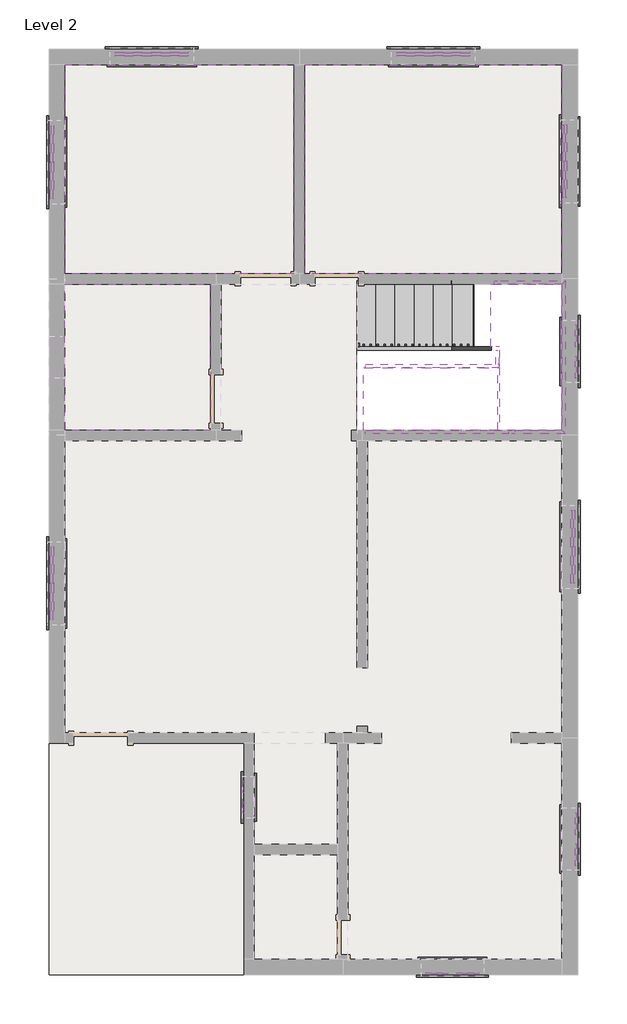
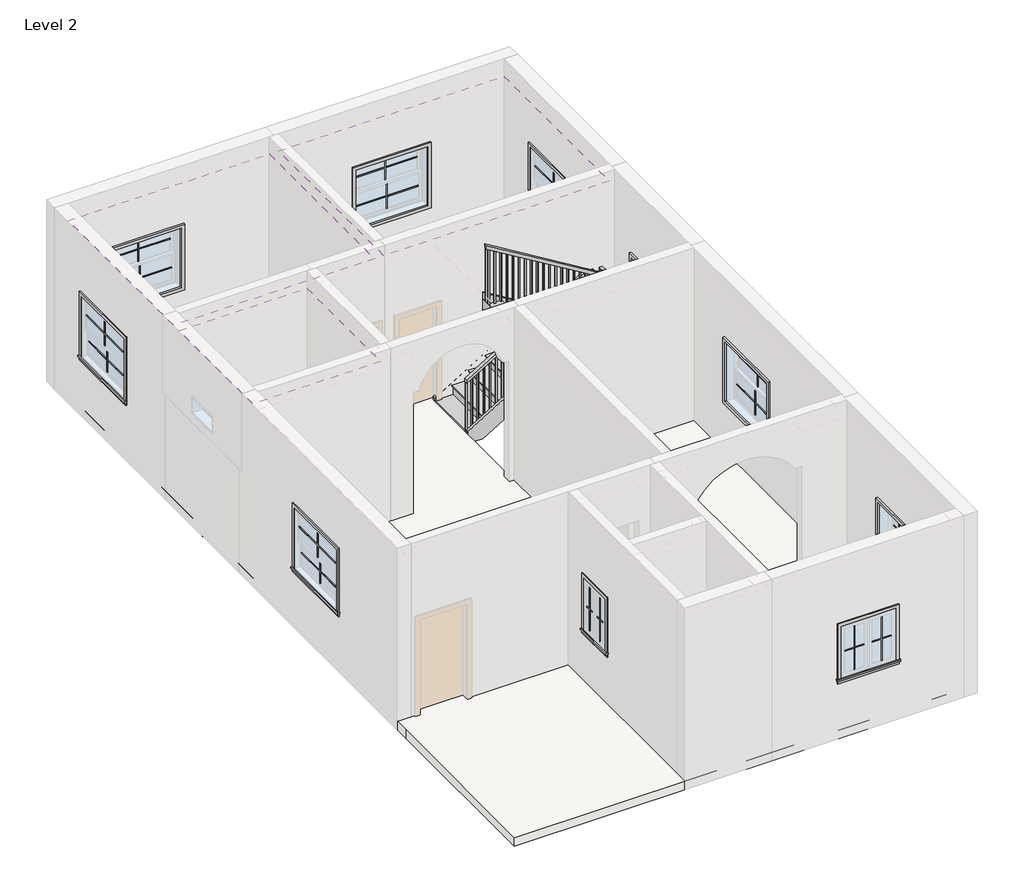
# One storey, part 2 of 2: 40 proxies, 8 members, 3 coverings, 2 slabs, 2 stair flights, 1 railing.
"""IFC4 building model written with IfcOpenShell, lengths in millimetres."""

from ifc_helpers import new_model, si_unit, frame, origin, place, context, project, spatial, polyline, outline, extrude, faceted_brep, transform, mapped, element, save
from components import muntin_pattern_2x2_muntin_pattern_2x2_8b3f23e7, muntin_pattern_2x2_muntin_pattern_2x2_5e52a1c6, muntin_pattern_2x2_muntin_pattern_2x2_d1c6e638, muntin_pattern_2x2_muntin_pattern_2x2_37b95fb2, muntin_pattern_2x2_muntin_pattern_2x2_53152e2c, muntin_pattern_2x2_muntin_pattern_2x2_e8f3e573, trim_window_exterior_flat_with_sill_f44f30ad, trim_window_exterior_flat_with_sill_e2e7eb1d, trim_window_exterior_flat_with_sill_84e24481, trim_window_exterior_flat_with_sill_a665a915, trim_window_interior_flat_picture_frame_1dce1945, trim_window_interior_flat_picture_frame_a40cb921, trim_window_interior_flat_picture_frame_28d4e5dc, trim_window_interior_flat_picture_frame_d485c387, non_monolithic_landing_52da1c58, stair_flight_171342da, stair_flight_f02a3465

model = new_model("IFC4")

# Units and contexts
model_context = context("Model", 3, world=origin())
ifc_project = project(units=[si_unit("LENGTHUNIT", "METRE", prefix="MILLI")], contexts=[model_context])

# Site, building, storey
site = spatial("IfcSite", under=ifc_project)
building = spatial("IfcBuilding", under=site)
storey = spatial("IfcBuildingStorey", under=building, Name="Level 2", Elevation=3200.4)

# Proxies
placement = place(None, origin())
muntin_pattern_2x2_muntin_pattern_2x2_shape = muntin_pattern_2x2_muntin_pattern_2x2_8b3f23e7(model_context)
element("IfcBuildingElementProxy", 1, Name="Muntin Pattern_2x2 : Muntin Pattern_2x2", ObjectType="Muntin Pattern_2x2 : Muntin Pattern_2x2", at=placement, inside=storey, context=model_context, shape_type="MappedRepresentation", body=[
    mapped(muntin_pattern_2x2_muntin_pattern_2x2_shape, transform((-5865.439062, 5032.1857363, 4975.225), x_axis=(0.0, 1.0, 0.0), y_axis=(-1.0, 0.0, 0.0), z_axis=(0.0, 0.0, 1.0))),
])
element("IfcBuildingElementProxy", 2, Name="Muntin Pattern_2x2 : Muntin Pattern_2x2", ObjectType="Muntin Pattern_2x2 : Muntin Pattern_2x2", at=placement, inside=storey, context=model_context, shape_type="MappedRepresentation", body=[
    mapped(muntin_pattern_2x2_muntin_pattern_2x2_shape, transform((-5820.989062, 5032.1857363, 4495.8), x_axis=(0.0, 1.0, 0.0), y_axis=(-1.0, 0.0, 0.0), z_axis=(0.0, 0.0, 1.0))),
])
element("IfcBuildingElementProxy", 3, Name="Muntin Pattern_2x2 : Muntin Pattern_2x2", ObjectType="Muntin Pattern_2x2 : Muntin Pattern_2x2", at=placement, inside=storey, context=model_context, shape_type="MappedRepresentation", body=[
    mapped(muntin_pattern_2x2_muntin_pattern_2x2_shape, transform((1786.310938, -581.2142637, 4975.225), x_axis=(0.0, -1.0, 0.0), y_axis=(1.0, 0.0, 0.0), z_axis=(0.0, 0.0, 1.0))),
])
element("IfcBuildingElementProxy", 4, Name="Muntin Pattern_2x2 : Muntin Pattern_2x2", ObjectType="Muntin Pattern_2x2 : Muntin Pattern_2x2", at=placement, inside=storey, context=model_context, shape_type="MappedRepresentation", body=[
    mapped(muntin_pattern_2x2_muntin_pattern_2x2_shape, transform((1741.860938, -581.2142637, 4495.8), x_axis=(0.0, -1.0, 0.0), y_axis=(1.0, 0.0, 0.0), z_axis=(0.0, 0.0, 1.0))),
])
element("IfcBuildingElementProxy", 5, Name="Muntin Pattern_2x2 : Muntin Pattern_2x2", ObjectType="Muntin Pattern_2x2 : Muntin Pattern_2x2", at=placement, inside=storey, context=model_context, shape_type="MappedRepresentation", body=[
    mapped(muntin_pattern_2x2_muntin_pattern_2x2_shape, transform((-5865.439062, -1114.6142637, 4975.225), x_axis=(0.0, 1.0, 0.0), y_axis=(-1.0, 0.0, 0.0), z_axis=(0.0, 0.0, 1.0))),
])
element("IfcBuildingElementProxy", 6, Name="Muntin Pattern_2x2 : Muntin Pattern_2x2", ObjectType="Muntin Pattern_2x2 : Muntin Pattern_2x2", at=placement, inside=storey, context=model_context, shape_type="MappedRepresentation", body=[
    mapped(muntin_pattern_2x2_muntin_pattern_2x2_shape, transform((-5820.989062, -1114.6142637, 4495.8), x_axis=(0.0, 1.0, 0.0), y_axis=(-1.0, 0.0, 0.0), z_axis=(0.0, 0.0, 1.0))),
])
muntin_pattern_2x2_muntin_pattern_2x2_2_shape = muntin_pattern_2x2_muntin_pattern_2x2_5e52a1c6(model_context)
element("IfcBuildingElementProxy", 7, Name="Muntin Pattern_2x2 : Muntin Pattern_2x2", ObjectType="Muntin Pattern_2x2 : Muntin Pattern_2x2", at=placement, inside=storey, context=model_context, shape_type="MappedRepresentation", body=[
    mapped(muntin_pattern_2x2_muntin_pattern_2x2_2_shape, transform((-4401.764062, 6648.2607363, 4975.225), x_axis=(-1.0, 0.0, 0.0), y_axis=(0.0, -1.0, 0.0), z_axis=(0.0, 0.0, 1.0))),
])
element("IfcBuildingElementProxy", 8, Name="Muntin Pattern_2x2 : Muntin Pattern_2x2", ObjectType="Muntin Pattern_2x2 : Muntin Pattern_2x2", at=placement, inside=storey, context=model_context, shape_type="MappedRepresentation", body=[
    mapped(muntin_pattern_2x2_muntin_pattern_2x2_2_shape, transform((-4401.764062, 6603.8107363, 4495.8), x_axis=(-1.0, 0.0, 0.0), y_axis=(0.0, -1.0, 0.0), z_axis=(0.0, 0.0, 1.0))),
])
element("IfcBuildingElementProxy", 9, Name="Muntin Pattern_2x2 : Muntin Pattern_2x2", ObjectType="Muntin Pattern_2x2 : Muntin Pattern_2x2", at=placement, inside=storey, context=model_context, shape_type="MappedRepresentation", body=[
    mapped(muntin_pattern_2x2_muntin_pattern_2x2_2_shape, transform((-286.964062, 6648.2607363, 4975.225), x_axis=(-1.0, 0.0, 0.0), y_axis=(0.0, -1.0, 0.0), z_axis=(0.0, 0.0, 1.0))),
])
element("IfcBuildingElementProxy", 10, Name="Muntin Pattern_2x2 : Muntin Pattern_2x2", ObjectType="Muntin Pattern_2x2 : Muntin Pattern_2x2", at=placement, inside=storey, context=model_context, shape_type="MappedRepresentation", body=[
    mapped(muntin_pattern_2x2_muntin_pattern_2x2_2_shape, transform((-286.964062, 6603.8107363, 4495.8), x_axis=(-1.0, 0.0, 0.0), y_axis=(0.0, -1.0, 0.0), z_axis=(0.0, 0.0, 1.0))),
])
element("IfcBuildingElementProxy", 11, Name="Muntin Pattern_2x2 : Muntin Pattern_2x2", ObjectType="Muntin Pattern_2x2 : Muntin Pattern_2x2", at=placement, inside=storey, context=model_context, shape_type="MappedRepresentation", body=[
    mapped(muntin_pattern_2x2_muntin_pattern_2x2_2_shape, transform((1627.560938, 5044.8857363, 4975.225), x_axis=(0.0, -1.0, 0.0), y_axis=(1.0, 0.0, 0.0), z_axis=(0.0, 0.0, 1.0))),
])
element("IfcBuildingElementProxy", 12, Name="Muntin Pattern_2x2 : Muntin Pattern_2x2", ObjectType="Muntin Pattern_2x2 : Muntin Pattern_2x2", at=placement, inside=storey, context=model_context, shape_type="MappedRepresentation", body=[
    mapped(muntin_pattern_2x2_muntin_pattern_2x2_2_shape, transform((1672.010938, 5044.8857363, 4495.8), x_axis=(0.0, -1.0, 0.0), y_axis=(1.0, 0.0, 0.0), z_axis=(0.0, 0.0, 1.0))),
])
muntin_pattern_2x2_muntin_pattern_2x2_3_shape = muntin_pattern_2x2_muntin_pattern_2x2_d1c6e638(model_context)
element("IfcBuildingElementProxy", 13, Name="Muntin Pattern_2x2 : Muntin Pattern_2x2", ObjectType="Muntin Pattern_2x2 : Muntin Pattern_2x2", at=placement, inside=storey, context=model_context, shape_type="MappedRepresentation", body=[
    mapped(muntin_pattern_2x2_muntin_pattern_2x2_3_shape, transform((1811.710938, -4621.4017637, 4489.45), x_axis=(0.0, -1.0, 0.0), y_axis=(1.0, 0.0, 0.0), z_axis=(0.0, 0.0, 1.0))),
])
element("IfcBuildingElementProxy", 14, Name="Muntin Pattern_2x2 : Muntin Pattern_2x2", ObjectType="Muntin Pattern_2x2 : Muntin Pattern_2x2", at=placement, inside=storey, context=model_context, shape_type="MappedRepresentation", body=[
    mapped(muntin_pattern_2x2_muntin_pattern_2x2_3_shape, transform((219.448438, -6820.0892637, 4489.45), x_axis=(-1.0, 0.0, 0.0), y_axis=(0.0, -1.0, 0.0), z_axis=(0.0, 0.0, 1.0))),
])
element("IfcBuildingElementProxy", 15, Name="Muntin Pattern_2x2 : Muntin Pattern_2x2", ObjectType="Muntin Pattern_2x2 : Muntin Pattern_2x2", at=placement, inside=storey, context=model_context, shape_type="MappedRepresentation", body=[
    mapped(muntin_pattern_2x2_muntin_pattern_2x2_3_shape, transform((1811.710938, 2496.9482363, 4489.45), x_axis=(0.0, -1.0, 0.0), y_axis=(1.0, 0.0, 0.0), z_axis=(0.0, 0.0, 1.0))),
])
muntin_pattern_2x2_muntin_pattern_2x2_4_shape = muntin_pattern_2x2_muntin_pattern_2x2_37b95fb2(model_context)
element("IfcBuildingElementProxy", 16, Name="Muntin Pattern_2x2 : Muntin Pattern_2x2", ObjectType="Muntin Pattern_2x2 : Muntin Pattern_2x2", at=placement, inside=storey, context=model_context, shape_type="MappedRepresentation", body=[
    mapped(muntin_pattern_2x2_muntin_pattern_2x2_4_shape, transform((1811.710938, -5075.4267637, 4489.45), x_axis=(0.0, 1.0, 0.0), y_axis=(-1.0, 0.0, 0.0), z_axis=(0.0, 0.0, 1.0))),
])
element("IfcBuildingElementProxy", 17, Name="Muntin Pattern_2x2 : Muntin Pattern_2x2", ObjectType="Muntin Pattern_2x2 : Muntin Pattern_2x2", at=placement, inside=storey, context=model_context, shape_type="MappedRepresentation", body=[
    mapped(muntin_pattern_2x2_muntin_pattern_2x2_4_shape, transform((-234.576562, -6820.0892637, 4489.45), x_axis=(1.0, 0.0, 0.0), y_axis=(0.0, 1.0, 0.0), z_axis=(0.0, 0.0, 1.0))),
])
element("IfcBuildingElementProxy", 18, Name="Muntin Pattern_2x2 : Muntin Pattern_2x2", ObjectType="Muntin Pattern_2x2 : Muntin Pattern_2x2", at=placement, inside=storey, context=model_context, shape_type="MappedRepresentation", body=[
    mapped(muntin_pattern_2x2_muntin_pattern_2x2_4_shape, transform((1811.710938, 2042.9232363, 4489.45), x_axis=(0.0, 1.0, 0.0), y_axis=(-1.0, 0.0, 0.0), z_axis=(0.0, 0.0, 1.0))),
])
muntin_pattern_2x2_muntin_pattern_2x2_5_shape = muntin_pattern_2x2_muntin_pattern_2x2_53152e2c(model_context)
element("IfcBuildingElementProxy", 19, Name="Muntin Pattern_2x2 : Muntin Pattern_2x2", ObjectType="Muntin Pattern_2x2 : Muntin Pattern_2x2", at=placement, inside=storey, context=model_context, shape_type="MappedRepresentation", body=[
    mapped(muntin_pattern_2x2_muntin_pattern_2x2_5_shape, transform((-3046.039062, -4389.6267637, 4489.45), x_axis=(0.0, 1.0, 0.0), y_axis=(-1.0, 0.0, 0.0), z_axis=(0.0, 0.0, 1.0))),
])
muntin_pattern_2x2_muntin_pattern_2x2_6_shape = muntin_pattern_2x2_muntin_pattern_2x2_e8f3e573(model_context)
element("IfcBuildingElementProxy", 20, Name="Muntin Pattern_2x2 : Muntin Pattern_2x2", ObjectType="Muntin Pattern_2x2 : Muntin Pattern_2x2", at=placement, inside=storey, context=model_context, shape_type="MappedRepresentation", body=[
    mapped(muntin_pattern_2x2_muntin_pattern_2x2_6_shape, transform((-3046.039062, -4088.0017637, 4489.45), x_axis=(0.0, -1.0, 0.0), y_axis=(1.0, 0.0, 0.0), z_axis=(0.0, 0.0, 1.0))),
])
trim_window_exterior_flat_with_sill_shape = trim_window_exterior_flat_with_sill_f44f30ad(model_context)
element("IfcBuildingElementProxy", 21, Name="Trim-Window-Exterior-Flat : with Sill", ObjectType="Trim-Window-Exterior-Flat : with Sill", at=placement, inside=storey, context=model_context, shape_type="MappedRepresentation", body=[
    mapped(trim_window_exterior_flat_with_sill_shape, transform((-5900.364062, 5032.1857363, 5486.4), x_axis=(0.0, -1.0, 0.0), y_axis=(0.0, 0.0, 1.0), z_axis=(-1.0, 0.0, 0.0))),
])
element("IfcBuildingElementProxy", 22, Name="Trim-Window-Exterior-Flat : with Sill", ObjectType="Trim-Window-Exterior-Flat : with Sill", at=placement, inside=storey, context=model_context, shape_type="MappedRepresentation", body=[
    mapped(trim_window_exterior_flat_with_sill_shape, transform((1821.235938, -581.2142637, 5486.4), x_axis=(0.0, 1.0, 0.0), y_axis=(0.0, 0.0, 1.0), z_axis=(1.0, 0.0, 0.0))),
])
element("IfcBuildingElementProxy", 23, Name="Trim-Window-Exterior-Flat : with Sill", ObjectType="Trim-Window-Exterior-Flat : with Sill", at=placement, inside=storey, context=model_context, shape_type="MappedRepresentation", body=[
    mapped(trim_window_exterior_flat_with_sill_shape, transform((-5900.364062, -1114.6142637, 5486.4), x_axis=(0.0, -1.0, 0.0), y_axis=(0.0, 0.0, 1.0), z_axis=(-1.0, 0.0, 0.0))),
])
trim_window_exterior_flat_with_sill_2_shape = trim_window_exterior_flat_with_sill_e2e7eb1d(model_context)
element("IfcBuildingElementProxy", 24, Name="Trim-Window-Exterior-Flat : with Sill", ObjectType="Trim-Window-Exterior-Flat : with Sill", at=placement, inside=storey, context=model_context, shape_type="MappedRepresentation", body=[
    mapped(trim_window_exterior_flat_with_sill_2_shape, transform((-4401.764062, 6683.1857363, 5486.4), x_axis=(1.0, 0.0, 0.0), y_axis=(0.0, 0.0, -1.0), z_axis=(0.0, 1.0, 0.0))),
])
element("IfcBuildingElementProxy", 25, Name="Trim-Window-Exterior-Flat : with Sill", ObjectType="Trim-Window-Exterior-Flat : with Sill", at=placement, inside=storey, context=model_context, shape_type="MappedRepresentation", body=[
    mapped(trim_window_exterior_flat_with_sill_2_shape, transform((-286.964062, 6683.1857363, 5486.4), x_axis=(1.0, 0.0, 0.0), y_axis=(0.0, 0.0, -1.0), z_axis=(0.0, 1.0, 0.0))),
])
element("IfcBuildingElementProxy", 26, Name="Trim-Window-Exterior-Flat : with Sill", ObjectType="Trim-Window-Exterior-Flat : with Sill", at=placement, inside=storey, context=model_context, shape_type="MappedRepresentation", body=[
    mapped(trim_window_exterior_flat_with_sill_2_shape, transform((1592.635938, 5044.8857363, 5486.4), x_axis=(0.0, 1.0, 0.0), y_axis=(0.0, 0.0, -1.0), z_axis=(-1.0, 0.0, 0.0))),
])
trim_window_exterior_flat_with_sill_3_shape = trim_window_exterior_flat_with_sill_84e24481(model_context)
element("IfcBuildingElementProxy", 27, Name="Trim-Window-Exterior-Flat : with Sill", ObjectType="Trim-Window-Exterior-Flat : with Sill", at=placement, inside=storey, context=model_context, shape_type="MappedRepresentation", body=[
    mapped(trim_window_exterior_flat_with_sill_3_shape, transform((1821.235938, -4848.4142637, 5334.0), x_axis=(0.0, 1.0, 0.0), y_axis=(0.0, 0.0, 1.0), z_axis=(1.0, 0.0, 0.0))),
])
element("IfcBuildingElementProxy", 28, Name="Trim-Window-Exterior-Flat : with Sill", ObjectType="Trim-Window-Exterior-Flat : with Sill", at=placement, inside=storey, context=model_context, shape_type="MappedRepresentation", body=[
    mapped(trim_window_exterior_flat_with_sill_3_shape, transform((-7.564062, -6829.6142637, 5334.0), x_axis=(1.0, 0.0, 0.0), y_axis=(0.0, 0.0, 1.0), z_axis=(0.0, -1.0, 0.0))),
])
element("IfcBuildingElementProxy", 29, Name="Trim-Window-Exterior-Flat : with Sill", ObjectType="Trim-Window-Exterior-Flat : with Sill", at=placement, inside=storey, context=model_context, shape_type="MappedRepresentation", body=[
    mapped(trim_window_exterior_flat_with_sill_3_shape, transform((1821.235938, 2269.9357363, 5334.0), x_axis=(0.0, 1.0, 0.0), y_axis=(0.0, 0.0, 1.0), z_axis=(1.0, 0.0, 0.0))),
])
trim_window_exterior_flat_with_sill_4_shape = trim_window_exterior_flat_with_sill_a665a915(model_context)
element("IfcBuildingElementProxy", 30, Name="Trim-Window-Exterior-Flat : with Sill", ObjectType="Trim-Window-Exterior-Flat : with Sill", at=placement, inside=storey, context=model_context, shape_type="MappedRepresentation", body=[
    mapped(trim_window_exterior_flat_with_sill_4_shape, transform((-3055.564062, -4238.8142637, 5334.0), x_axis=(0.0, -1.0, 0.0), y_axis=(0.0, 0.0, 1.0), z_axis=(-1.0, 0.0, 0.0))),
])
trim_window_interior_flat_picture_frame_shape = trim_window_interior_flat_picture_frame_1dce1945(model_context)
element("IfcBuildingElementProxy", 31, Name="Trim-Window-Interior-Flat : Picture Frame", ObjectType="Trim-Window-Interior-Flat : Picture Frame", at=placement, inside=storey, context=model_context, shape_type="MappedRepresentation", body=[
    mapped(trim_window_interior_flat_picture_frame_shape, transform((-5671.764062, 5032.1857363, 5486.4), x_axis=(0.0, 1.0, 0.0), y_axis=(0.0, 0.0, 1.0), z_axis=(1.0, 0.0, 0.0))),
])
element("IfcBuildingElementProxy", 32, Name="Trim-Window-Interior-Flat : Picture Frame", ObjectType="Trim-Window-Interior-Flat : Picture Frame", at=placement, inside=storey, context=model_context, shape_type="MappedRepresentation", body=[
    mapped(trim_window_interior_flat_picture_frame_shape, transform((1592.635938, -581.2142637, 5486.4), x_axis=(0.0, -1.0, 0.0), y_axis=(0.0, 0.0, 1.0), z_axis=(-1.0, 0.0, 0.0))),
])
element("IfcBuildingElementProxy", 33, Name="Trim-Window-Interior-Flat : Picture Frame", ObjectType="Trim-Window-Interior-Flat : Picture Frame", at=placement, inside=storey, context=model_context, shape_type="MappedRepresentation", body=[
    mapped(trim_window_interior_flat_picture_frame_shape, transform((-5671.764062, -1114.6142637, 5486.4), x_axis=(0.0, 1.0, 0.0), y_axis=(0.0, 0.0, 1.0), z_axis=(1.0, 0.0, 0.0))),
])
trim_window_interior_flat_picture_frame_2_shape = trim_window_interior_flat_picture_frame_a40cb921(model_context)
element("IfcBuildingElementProxy", 34, Name="Trim-Window-Interior-Flat : Picture Frame", ObjectType="Trim-Window-Interior-Flat : Picture Frame", at=placement, inside=storey, context=model_context, shape_type="MappedRepresentation", body=[
    mapped(trim_window_interior_flat_picture_frame_2_shape, transform((-4401.764062, 6454.5857363, 5486.4), x_axis=(-1.0, 0.0, 0.0), y_axis=(0.0, 0.0, -1.0), z_axis=(0.0, -1.0, 0.0))),
])
element("IfcBuildingElementProxy", 35, Name="Trim-Window-Interior-Flat : Picture Frame", ObjectType="Trim-Window-Interior-Flat : Picture Frame", at=placement, inside=storey, context=model_context, shape_type="MappedRepresentation", body=[
    mapped(trim_window_interior_flat_picture_frame_2_shape, transform((-286.964062, 6454.5857363, 5486.4), x_axis=(-1.0, 0.0, 0.0), y_axis=(0.0, 0.0, -1.0), z_axis=(0.0, -1.0, 0.0))),
])
element("IfcBuildingElementProxy", 36, Name="Trim-Window-Interior-Flat : Picture Frame", ObjectType="Trim-Window-Interior-Flat : Picture Frame", at=placement, inside=storey, context=model_context, shape_type="MappedRepresentation", body=[
    mapped(trim_window_interior_flat_picture_frame_2_shape, transform((1821.235938, 5044.8857363, 5486.4), x_axis=(0.0, -1.0, 0.0), y_axis=(0.0, 0.0, -1.0), z_axis=(1.0, 0.0, 0.0))),
])
trim_window_interior_flat_picture_frame_3_shape = trim_window_interior_flat_picture_frame_28d4e5dc(model_context)
element("IfcBuildingElementProxy", 37, Name="Trim-Window-Interior-Flat : Picture Frame", ObjectType="Trim-Window-Interior-Flat : Picture Frame", at=placement, inside=storey, context=model_context, shape_type="MappedRepresentation", body=[
    mapped(trim_window_interior_flat_picture_frame_3_shape, transform((1592.635938, -4848.4142637, 5334.0), x_axis=(0.0, -1.0, 0.0), y_axis=(0.0, 0.0, 1.0), z_axis=(-1.0, 0.0, 0.0))),
])
element("IfcBuildingElementProxy", 38, Name="Trim-Window-Interior-Flat : Picture Frame", ObjectType="Trim-Window-Interior-Flat : Picture Frame", at=placement, inside=storey, context=model_context, shape_type="MappedRepresentation", body=[
    mapped(trim_window_interior_flat_picture_frame_3_shape, transform((-7.564062, -6601.0142637, 5334.0), x_axis=(-1.0, 0.0, 0.0), y_axis=(0.0, 0.0, 1.0), z_axis=(0.0, 1.0, 0.0))),
])
element("IfcBuildingElementProxy", 39, Name="Trim-Window-Interior-Flat : Picture Frame", ObjectType="Trim-Window-Interior-Flat : Picture Frame", at=placement, inside=storey, context=model_context, shape_type="MappedRepresentation", body=[
    mapped(trim_window_interior_flat_picture_frame_3_shape, transform((1592.635938, 2269.9357363, 5334.0), x_axis=(0.0, -1.0, 0.0), y_axis=(0.0, 0.0, 1.0), z_axis=(-1.0, 0.0, 0.0))),
])
trim_window_interior_flat_picture_frame_4_shape = trim_window_interior_flat_picture_frame_d485c387(model_context)
element("IfcBuildingElementProxy", 40, Name="Trim-Window-Interior-Flat : Picture Frame", ObjectType="Trim-Window-Interior-Flat : Picture Frame", at=placement, inside=storey, context=model_context, shape_type="MappedRepresentation", body=[
    mapped(trim_window_interior_flat_picture_frame_4_shape, transform((-2903.164062, -4238.8142637, 5334.0), x_axis=(0.0, 1.0, 0.0), y_axis=(0.0, 0.0, 1.0), z_axis=(1.0, 0.0, 0.0))),
])

# Coverings
element("IfcCovering", 41, ObjectType="2' x 4' ACT System", at=placement, inside=storey, context=model_context, shape_type="SweptSolid", body=[
    extrude(outline(polyline([(-5671.764062, 3406.5857363), (-5671.764062, 6454.5857363), (-2318.964062, 6454.5857363), (-2318.964062, 3406.5857363), (-3461.964062, 3406.5857363), (-5671.764062, 3406.5857363)])), frame((0.0, 0.0, 6248.4), z_axis=(0.0, 0.0, 1.0), x_axis=(1.0, 0.0, 0.0)), (0.0, 0.0, 1.0), 57.15),
])
element("IfcCovering", 42, ObjectType="2' x 4' ACT System", at=placement, inside=storey, context=model_context, shape_type="SweptSolid", body=[
    extrude(outline(polyline([(1592.635938, 6454.5857363), (1592.635938, 3406.5857363), (-2166.564062, 3406.5857363), (-2166.564062, 6454.5857363), (1592.635938, 6454.5857363)])), frame((0.0, 0.0, 6248.4), z_axis=(0.0, 0.0, 1.0), x_axis=(1.0, 0.0, 0.0)), (0.0, 0.0, 1.0), 57.15),
])
element("IfcCovering", 43, ObjectType="2' x 4' ACT System", at=placement, inside=storey, context=model_context, shape_type="SweptSolid", body=[
    extrude(outline(polyline([(-5671.764062, 1120.5857363), (-5671.764062, 3254.1857363), (-3538.164062, 3254.1857363), (-3538.164062, 1120.5857363), (-5671.764062, 1120.5857363)])), frame((0.0, 0.0, 6248.4), z_axis=(0.0, 0.0, 1.0), x_axis=(1.0, 0.0, 0.0)), (0.0, 0.0, 1.0), 57.15),
])

# Members
element("IfcMember", 44, ObjectType="Stringer - 2\" Width", at=placement, inside=storey, context=model_context, shape_type="SweptSolid", body=[
    extrude(outline(polyline([(3564.914512, -1404.564062), (3352.8, -1404.564062), (3352.8, -1166.4785503), (4478.8666667, 691.5314497), (4783.6666667, 606.3769932), (3564.914512, -1404.564062)])), frame((0.0, 3254.1857363, 0.0), z_axis=(0.0, 1.0, 0.0), x_axis=(0.0, 0.0, 1.0)), (0.0, 0.0, 1.0), 50.8),
])
element("IfcMember", 45, ObjectType="Stringer - 2\" Width", at=placement, inside=storey, context=model_context, shape_type="SweptSolid", body=[
    extrude(outline(polyline([(3564.914512, -1404.564062), (3352.8, -1404.564062), (3352.8, -1166.4785503), (4470.8087807, 678.235938), (4783.6666667, 678.235938), (4783.6666667, 606.3769932), (3564.914512, -1404.564062)])), frame((0.0, 2288.9857363, 0.0), z_axis=(0.0, 1.0, 0.0), x_axis=(0.0, 0.0, 1.0)), (0.0, 0.0, 1.0), 50.8),
])
element("IfcMember", 46, ObjectType="Stringer - 2\" Width", at=placement, inside=storey, context=model_context, shape_type="SweptSolid", body=[
    extrude(outline(polyline([(4478.8666667, 817.3404262), (4783.6666667, 902.4948827), (6104.914512, -1277.564062), (5748.5057504, -1277.564062), (4478.8666667, 817.3404262)])), frame((0.0, 1069.7857363, 0.0), z_axis=(0.0, 1.0, 0.0), x_axis=(0.0, 0.0, 1.0)), (0.0, 0.0, 1.0), 50.8),
])
element("IfcMember", 47, ObjectType="Stringer - 2\" Width", at=placement, inside=storey, context=model_context, shape_type="SweptSolid", body=[
    extrude(outline(polyline([(4563.1724171, 678.235938), (4919.5811786, 678.235938), (6104.914512, -1277.564062), (5748.5057504, -1277.564062), (4563.1724171, 678.235938)])), frame((0.0, 2034.9857363, 0.0), z_axis=(0.0, 1.0, 0.0), x_axis=(0.0, 0.0, 1.0)), (0.0, 0.0, 1.0), 50.8),
])
element("IfcMember", 48, ObjectType="Stringer - 2\" Width", at=placement, inside=storey, context=model_context, shape_type="Brep", body=[
    faceted_brep([(902.4948827, 1120.5857363, 4783.6666667), (902.4948827, 1069.7857363, 4783.6666667), (1643.435938, 1069.7857363, 4783.6666667), (1592.635938, 1120.5857363, 4783.6666667), (817.3404262, 1120.5857363, 4478.8666667), (1592.635938, 1120.5857363, 4478.8666667), (817.3404262, 1069.7857363, 4478.8666667), (1643.435938, 1069.7857363, 4478.8666667)], [[[0, 1, 2, 3]], [[4, 0, 3, 5]], [[6, 4, 5, 7]], [[1, 6, 7, 2]], [[1, 0, 4, 6]], [[2, 7, 5, 3]]]),
])
element("IfcMember", 49, ObjectType="Stringer - 2\" Width", at=placement, inside=storey, context=model_context, shape_type="SweptSolid", body=[
    extrude(outline(polyline([(1643.435938, 1069.7857363), (1592.635938, 1120.5857363), (1592.635938, 3254.1857363), (1643.435938, 3304.9857363), (1643.435938, 1069.7857363)])), frame((0.0, 0.0, 4478.8666667), z_axis=(0.0, 0.0, 1.0), x_axis=(1.0, 0.0, 0.0)), (0.0, 0.0, 1.0), 304.8),
])
element("IfcMember", 50, ObjectType="Stringer - 2\" Width", at=placement, inside=storey, context=model_context, shape_type="Brep", body=[
    faceted_brep([(1592.635938, 3254.1857363, 4783.6666667), (1643.435938, 3304.9857363, 4783.6666667), (606.3769932, 3304.9857363, 4783.6666667), (606.3769932, 3254.1857363, 4783.6666667), (1592.635938, 3254.1857363, 4478.8666667), (691.5314497, 3254.1857363, 4478.8666667), (1643.435938, 3304.9857363, 4478.8666667), (691.5314497, 3304.9857363, 4478.8666667)], [[[0, 1, 2, 3]], [[4, 0, 3, 5]], [[6, 4, 5, 7]], [[1, 6, 7, 2]], [[1, 0, 4, 6]], [[2, 7, 5, 3]]]),
])
element("IfcMember", 51, ObjectType="Stringer - 2\" Width", at=placement, inside=storey, context=model_context, shape_type="SweptSolid", body=[
    extrude(outline(polyline([(627.435938, 2288.9857363), (678.235938, 2288.9857363), (678.235938, 2085.7857363), (627.435938, 2085.7857363), (627.435938, 2288.9857363)])), frame((0.0, 0.0, 4478.8666667), z_axis=(0.0, 0.0, 1.0), x_axis=(1.0, 0.0, 0.0)), (0.0, 0.0, 1.0), 304.8),
])

# Railing
element("IfcRailing", 52, ObjectType="Handrail - Rectangular", at=placement, inside=storey, context=model_context, shape_type="SolidModel", body=[
    faceted_brep([(-1404.564062, 2390.5857363, 4436.5333333), (-1404.564062, 2390.5857363, 4377.1318731), (-1404.564062, 2339.7857363, 4377.1318731), (-1404.564062, 2339.7857363, 4436.5333333), (551.235938, 2390.5857363, 5621.8666667), (565.4283474, 2390.5857363, 5571.0666667), (565.4283474, 2339.7857363, 5571.0666667), (551.235938, 2339.7857363, 5621.8666667), (729.035938, 2390.5857363, 5621.8666667), (729.035938, 2390.5857363, 5571.0666667), (678.235938, 2339.7857363, 5571.0666667), (678.235938, 2339.7857363, 5621.8666667), (729.035938, 2111.1857363, 5621.8666667), (729.035938, 2060.3857363, 5571.0666667), (678.235938, 2060.3857363, 5571.0666667), (678.235938, 2111.1857363, 5621.8666667), (729.035938, 2111.1857363, 5837.3818182), (729.035938, 2060.3857363, 5786.5818182), (678.235938, 2060.3857363, 5786.5818182), (678.235938, 2111.1857363, 5837.3818182), (729.035938, 1984.1857363, 5837.3818182), (729.035938, 1984.1857363, 5786.5818182), (678.235938, 2034.9857363, 5786.5818182), (678.235938, 2034.9857363, 5837.3818182), (602.035938, 1984.1857363, 5837.3818182), (587.8435285, 1984.1857363, 5786.5818182), (587.8435285, 2034.9857363, 5786.5818182), (602.035938, 2034.9857363, 5837.3818182), (-1277.564062, 1984.1857363, 6976.5333333), (-1277.564062, 2034.9857363, 6976.5333333), (-1277.564062, 2034.9857363, 6917.1318731), (-1277.564062, 1984.1857363, 6917.1318731)], [[[0, 1, 2, 3]], [[1, 0, 4, 5]], [[2, 1, 5, 6]], [[3, 2, 6, 7]], [[0, 3, 7, 4]], [[5, 4, 8, 9]], [[6, 5, 9, 10]], [[7, 6, 10, 11]], [[4, 7, 11, 8]], [[9, 8, 12, 13]], [[10, 9, 13, 14]], [[11, 10, 14, 15]], [[8, 11, 15, 12]], [[13, 12, 16, 17]], [[14, 13, 17, 18]], [[15, 14, 18, 19]], [[12, 15, 19, 16]], [[17, 16, 20, 21]], [[18, 17, 21, 22]], [[19, 18, 22, 23]], [[16, 19, 23, 20]], [[21, 20, 24, 25]], [[22, 21, 25, 26]], [[23, 22, 26, 27]], [[20, 23, 27, 24]], [[28, 29, 30, 31]], [[25, 24, 28, 31]], [[26, 25, 31, 30]], [[27, 26, 30, 29]], [[24, 27, 29, 28]]]),
    extrude(outline(polyline([(6880.571267, -1217.239062), (6892.1167216, -1236.289062), (5892.8, -1236.289062), (5892.8, -1217.239062), (6880.571267, -1217.239062)])), frame((0.0, 2000.0607363, 0.0), z_axis=(0.0, 1.0, 0.0), x_axis=(0.0, 0.0, 1.0)), (0.0, 0.0, 1.0), 19.05),
    extrude(outline(polyline([(6818.9955094, -1115.639062), (6830.540964, -1134.689062), (5892.8, -1134.689062), (5892.8, -1115.639062), (6818.9955094, -1115.639062)])), frame((0.0, 2000.0607363, 0.0), z_axis=(0.0, 1.0, 0.0), x_axis=(0.0, 0.0, 1.0)), (0.0, 0.0, 1.0), 19.05),
    extrude(outline(polyline([(6757.4197519, -1014.039062), (6768.9652064, -1033.089062), (5892.8, -1033.089062), (5892.8, -1014.039062), (6757.4197519, -1014.039062)])), frame((0.0, 2000.0607363, 0.0), z_axis=(0.0, 1.0, 0.0), x_axis=(0.0, 0.0, 1.0)), (0.0, 0.0, 1.0), 19.05),
    extrude(outline(polyline([(6695.8439943, -912.439062), (6707.3894488, -931.489062), (5723.4666667, -931.489062), (5723.4666667, -912.439062), (6695.8439943, -912.439062)])), frame((0.0, 2000.0607363, 0.0), z_axis=(0.0, 1.0, 0.0), x_axis=(0.0, 0.0, 1.0)), (0.0, 0.0, 1.0), 19.05),
    extrude(outline(polyline([(6634.2682367, -810.839062), (6645.8136913, -829.889062), (5723.4666667, -829.889062), (5723.4666667, -810.839062), (6634.2682367, -810.839062)])), frame((0.0, 2000.0607363, 0.0), z_axis=(0.0, 1.0, 0.0), x_axis=(0.0, 0.0, 1.0)), (0.0, 0.0, 1.0), 19.05),
    extrude(outline(polyline([(6572.6924791, -709.239062), (6584.2379337, -728.289062), (5723.4666667, -728.289062), (5723.4666667, -709.239062), (6572.6924791, -709.239062)])), frame((0.0, 2000.0607363, 0.0), z_axis=(0.0, 1.0, 0.0), x_axis=(0.0, 0.0, 1.0)), (0.0, 0.0, 1.0), 19.05),
    extrude(outline(polyline([(6511.1167216, -607.639062), (6522.6621761, -626.689062), (5554.1333333, -626.689062), (5554.1333333, -607.639062), (6511.1167216, -607.639062)])), frame((0.0, 2000.0607363, 0.0), z_axis=(0.0, 1.0, 0.0), x_axis=(0.0, 0.0, 1.0)), (0.0, 0.0, 1.0), 19.05),
    extrude(outline(polyline([(6449.540964, -506.039062), (6461.0864185, -525.089062), (5554.1333333, -525.089062), (5554.1333333, -506.039062), (6449.540964, -506.039062)])), frame((0.0, 2000.0607363, 0.0), z_axis=(0.0, 1.0, 0.0), x_axis=(0.0, 0.0, 1.0)), (0.0, 0.0, 1.0), 19.05),
    extrude(outline(polyline([(6387.9652064, -404.439062), (6399.510661, -423.489062), (5384.8, -423.489062), (5384.8, -404.439062), (6387.9652064, -404.439062)])), frame((0.0, 2000.0607363, 0.0), z_axis=(0.0, 1.0, 0.0), x_axis=(0.0, 0.0, 1.0)), (0.0, 0.0, 1.0), 19.05),
    extrude(outline(polyline([(6326.3894488, -302.839062), (6337.9349034, -321.889062), (5384.8, -321.889062), (5384.8, -302.839062), (6326.3894488, -302.839062)])), frame((0.0, 2000.0607363, 0.0), z_axis=(0.0, 1.0, 0.0), x_axis=(0.0, 0.0, 1.0)), (0.0, 0.0, 1.0), 19.05),
    extrude(outline(polyline([(6264.8136913, -201.239062), (6276.3591458, -220.289062), (5384.8, -220.289062), (5384.8, -201.239062), (6264.8136913, -201.239062)])), frame((0.0, 2000.0607363, 0.0), z_axis=(0.0, 1.0, 0.0), x_axis=(0.0, 0.0, 1.0)), (0.0, 0.0, 1.0), 19.05),
    extrude(outline(polyline([(6203.2379337, -99.639062), (6214.7833882, -118.689062), (5215.4666667, -118.689062), (5215.4666667, -99.639062), (6203.2379337, -99.639062)])), frame((0.0, 2000.0607363, 0.0), z_axis=(0.0, 1.0, 0.0), x_axis=(0.0, 0.0, 1.0)), (0.0, 0.0, 1.0), 19.05),
    extrude(outline(polyline([(6141.6621761, 1.960938), (6153.2076307, -17.089062), (5215.4666667, -17.089062), (5215.4666667, 1.960938), (6141.6621761, 1.960938)])), frame((0.0, 2000.0607363, 0.0), z_axis=(0.0, 1.0, 0.0), x_axis=(0.0, 0.0, 1.0)), (0.0, 0.0, 1.0), 19.05),
    extrude(outline(polyline([(6080.0864185, 103.560938), (6091.6318731, 84.510938), (5215.4666667, 84.510938), (5215.4666667, 103.560938), (6080.0864185, 103.560938)])), frame((0.0, 2000.0607363, 0.0), z_axis=(0.0, 1.0, 0.0), x_axis=(0.0, 0.0, 1.0)), (0.0, 0.0, 1.0), 19.05),
    extrude(outline(polyline([(6018.510661, 205.160938), (6030.0561155, 186.110938), (5046.1333333, 186.110938), (5046.1333333, 205.160938), (6018.510661, 205.160938)])), frame((0.0, 2000.0607363, 0.0), z_axis=(0.0, 1.0, 0.0), x_axis=(0.0, 0.0, 1.0)), (0.0, 0.0, 1.0), 19.05),
    extrude(outline(polyline([(5956.9349034, 306.760938), (5968.4803579, 287.710938), (5046.1333333, 287.710938), (5046.1333333, 306.760938), (5956.9349034, 306.760938)])), frame((0.0, 2000.0607363, 0.0), z_axis=(0.0, 1.0, 0.0), x_axis=(0.0, 0.0, 1.0)), (0.0, 0.0, 1.0), 19.05),
    extrude(outline(polyline([(5895.3591458, 408.360938), (5906.9046004, 389.310938), (5046.1333333, 389.310938), (5046.1333333, 408.360938), (5895.3591458, 408.360938)])), frame((0.0, 2000.0607363, 0.0), z_axis=(0.0, 1.0, 0.0), x_axis=(0.0, 0.0, 1.0)), (0.0, 0.0, 1.0), 19.05),
    extrude(outline(polyline([(5833.7833882, 509.960938), (5845.3288428, 490.910938), (4876.8, 490.910938), (4876.8, 509.960938), (5833.7833882, 509.960938)])), frame((0.0, 2000.0607363, 0.0), z_axis=(0.0, 1.0, 0.0), x_axis=(0.0, 0.0, 1.0)), (0.0, 0.0, 1.0), 19.05),
    extrude(outline(polyline([(5772.2076307, 611.560938), (5783.7530852, 592.510938), (4876.8, 592.510938), (4876.8, 611.560938), (5772.2076307, 611.560938)])), frame((0.0, 2000.0607363, 0.0), z_axis=(0.0, 1.0, 0.0), x_axis=(0.0, 0.0, 1.0)), (0.0, 0.0, 1.0), 19.05),
    extrude(outline(polyline([(694.110938, 2069.9107363), (713.160938, 2069.9107363), (713.160938, 2050.8607363), (694.110938, 2050.8607363), (694.110938, 2069.9107363)])), frame((0.0, 0.0, 4707.4666667), z_axis=(0.0, 0.0, 1.0), x_axis=(1.0, 0.0, 0.0)), (0.0, 0.0, 1.0), 1079.1151515),
    extrude(outline(polyline([(694.110938, 2171.5107363), (713.160938, 2171.5107363), (713.160938, 2152.4607363), (694.110938, 2152.4607363), (694.110938, 2171.5107363)])), frame((0.0, 0.0, 4707.4666667), z_axis=(0.0, 0.0, 1.0), x_axis=(1.0, 0.0, 0.0)), (0.0, 0.0, 1.0), 863.6),
    extrude(outline(polyline([(694.110938, 2273.1107363), (713.160938, 2273.1107363), (713.160938, 2254.0607363), (694.110938, 2254.0607363), (694.110938, 2273.1107363)])), frame((0.0, 0.0, 4707.4666667), z_axis=(0.0, 0.0, 1.0), x_axis=(1.0, 0.0, 0.0)), (0.0, 0.0, 1.0), 863.6),
    extrude(outline(polyline([(643.310938, 2355.6607363), (643.310938, 2374.7107363), (662.360938, 2374.7107363), (662.360938, 2355.6607363), (643.310938, 2355.6607363)])), frame((0.0, 0.0, 4707.4666667), z_axis=(0.0, 0.0, 1.0), x_axis=(1.0, 0.0, 0.0)), (0.0, 0.0, 1.0), 863.6),
    extrude(outline(polyline([(5552.8439943, 535.360938), (5541.2985397, 516.310938), (4538.1333333, 516.310938), (4538.1333333, 535.360938), (5552.8439943, 535.360938)])), frame((0.0, 2355.6607363, 0.0), z_axis=(0.0, 1.0, 0.0), x_axis=(0.0, 0.0, 1.0)), (0.0, 0.0, 1.0), 19.05),
    extrude(outline(polyline([(5491.2682367, 433.760938), (5479.7227822, 414.710938), (4538.1333333, 414.710938), (4538.1333333, 433.760938), (5491.2682367, 433.760938)])), frame((0.0, 2355.6607363, 0.0), z_axis=(0.0, 1.0, 0.0), x_axis=(0.0, 0.0, 1.0)), (0.0, 0.0, 1.0), 19.05),
    extrude(outline(polyline([(5429.6924791, 332.160938), (5418.1470246, 313.110938), (4538.1333333, 313.110938), (4538.1333333, 332.160938), (5429.6924791, 332.160938)])), frame((0.0, 2355.6607363, 0.0), z_axis=(0.0, 1.0, 0.0), x_axis=(0.0, 0.0, 1.0)), (0.0, 0.0, 1.0), 19.05),
    extrude(outline(polyline([(5368.1167216, 230.560938), (5356.571267, 211.510938), (4368.8, 211.510938), (4368.8, 230.560938), (5368.1167216, 230.560938)])), frame((0.0, 2355.6607363, 0.0), z_axis=(0.0, 1.0, 0.0), x_axis=(0.0, 0.0, 1.0)), (0.0, 0.0, 1.0), 19.05),
    extrude(outline(polyline([(5306.540964, 128.960938), (5294.9955094, 109.910938), (4368.8, 109.910938), (4368.8, 128.960938), (5306.540964, 128.960938)])), frame((0.0, 2355.6607363, 0.0), z_axis=(0.0, 1.0, 0.0), x_axis=(0.0, 0.0, 1.0)), (0.0, 0.0, 1.0), 19.05),
    extrude(outline(polyline([(5244.9652064, 27.360938), (5233.4197519, 8.310938), (4368.8, 8.310938), (4368.8, 27.360938), (5244.9652064, 27.360938)])), frame((0.0, 2355.6607363, 0.0), z_axis=(0.0, 1.0, 0.0), x_axis=(0.0, 0.0, 1.0)), (0.0, 0.0, 1.0), 19.05),
    extrude(outline(polyline([(5183.3894488, -74.239062), (5171.8439943, -93.289062), (4199.4666667, -93.289062), (4199.4666667, -74.239062), (5183.3894488, -74.239062)])), frame((0.0, 2355.6607363, 0.0), z_axis=(0.0, 1.0, 0.0), x_axis=(0.0, 0.0, 1.0)), (0.0, 0.0, 1.0), 19.05),
    extrude(outline(polyline([(5121.8136913, -175.839062), (5110.2682367, -194.889062), (4199.4666667, -194.889062), (4199.4666667, -175.839062), (5121.8136913, -175.839062)])), frame((0.0, 2355.6607363, 0.0), z_axis=(0.0, 1.0, 0.0), x_axis=(0.0, 0.0, 1.0)), (0.0, 0.0, 1.0), 19.05),
    extrude(outline(polyline([(5060.2379337, -277.439062), (5048.6924791, -296.489062), (4199.4666667, -296.489062), (4199.4666667, -277.439062), (5060.2379337, -277.439062)])), frame((0.0, 2355.6607363, 0.0), z_axis=(0.0, 1.0, 0.0), x_axis=(0.0, 0.0, 1.0)), (0.0, 0.0, 1.0), 19.05),
    extrude(outline(polyline([(4998.6621761, -379.039062), (4987.1167216, -398.089062), (4030.1333333, -398.089062), (4030.1333333, -379.039062), (4998.6621761, -379.039062)])), frame((0.0, 2355.6607363, 0.0), z_axis=(0.0, 1.0, 0.0), x_axis=(0.0, 0.0, 1.0)), (0.0, 0.0, 1.0), 19.05),
    extrude(outline(polyline([(4937.0864185, -480.639062), (4925.540964, -499.689062), (4030.1333333, -499.689062), (4030.1333333, -480.639062), (4937.0864185, -480.639062)])), frame((0.0, 2355.6607363, 0.0), z_axis=(0.0, 1.0, 0.0), x_axis=(0.0, 0.0, 1.0)), (0.0, 0.0, 1.0), 19.05),
    extrude(outline(polyline([(4875.510661, -582.239062), (4863.9652064, -601.289062), (3860.8, -601.289062), (3860.8, -582.239062), (4875.510661, -582.239062)])), frame((0.0, 2355.6607363, 0.0), z_axis=(0.0, 1.0, 0.0), x_axis=(0.0, 0.0, 1.0)), (0.0, 0.0, 1.0), 19.05),
    extrude(outline(polyline([(4813.9349034, -683.839062), (4802.3894488, -702.889062), (3860.8, -702.889062), (3860.8, -683.839062), (4813.9349034, -683.839062)])), frame((0.0, 2355.6607363, 0.0), z_axis=(0.0, 1.0, 0.0), x_axis=(0.0, 0.0, 1.0)), (0.0, 0.0, 1.0), 19.05),
    extrude(outline(polyline([(4752.3591458, -785.439062), (4740.8136913, -804.489062), (3860.8, -804.489062), (3860.8, -785.439062), (4752.3591458, -785.439062)])), frame((0.0, 2355.6607363, 0.0), z_axis=(0.0, 1.0, 0.0), x_axis=(0.0, 0.0, 1.0)), (0.0, 0.0, 1.0), 19.05),
    extrude(outline(polyline([(4690.7833882, -887.039062), (4679.2379337, -906.089062), (3691.4666667, -906.089062), (3691.4666667, -887.039062), (4690.7833882, -887.039062)])), frame((0.0, 2355.6607363, 0.0), z_axis=(0.0, 1.0, 0.0), x_axis=(0.0, 0.0, 1.0)), (0.0, 0.0, 1.0), 19.05),
    extrude(outline(polyline([(4629.2076307, -988.639062), (4617.6621761, -1007.689062), (3691.4666667, -1007.689062), (3691.4666667, -988.639062), (4629.2076307, -988.639062)])), frame((0.0, 2355.6607363, 0.0), z_axis=(0.0, 1.0, 0.0), x_axis=(0.0, 0.0, 1.0)), (0.0, 0.0, 1.0), 19.05),
    extrude(outline(polyline([(4567.6318731, -1090.239062), (4556.0864185, -1109.289062), (3691.4666667, -1109.289062), (3691.4666667, -1090.239062), (4567.6318731, -1090.239062)])), frame((0.0, 2355.6607363, 0.0), z_axis=(0.0, 1.0, 0.0), x_axis=(0.0, 0.0, 1.0)), (0.0, 0.0, 1.0), 19.05),
    extrude(outline(polyline([(4506.0561155, -1191.839062), (4494.510661, -1210.889062), (3522.1333333, -1210.889062), (3522.1333333, -1191.839062), (4506.0561155, -1191.839062)])), frame((0.0, 2355.6607363, 0.0), z_axis=(0.0, 1.0, 0.0), x_axis=(0.0, 0.0, 1.0)), (0.0, 0.0, 1.0), 19.05),
    extrude(outline(polyline([(4444.4803579, -1293.439062), (4432.9349034, -1312.489062), (3522.1333333, -1312.489062), (3522.1333333, -1293.439062), (4444.4803579, -1293.439062)])), frame((0.0, 2355.6607363, 0.0), z_axis=(0.0, 1.0, 0.0), x_axis=(0.0, 0.0, 1.0)), (0.0, 0.0, 1.0), 19.05),
    extrude(outline(polyline([(694.110938, 2019.1107363), (713.160938, 2019.1107363), (713.160938, 2000.0607363), (694.110938, 2000.0607363), (694.110938, 2019.1107363)])), frame((0.0, 0.0, 4707.4666667), z_axis=(0.0, 0.0, 1.0), x_axis=(1.0, 0.0, 0.0)), (0.0, 0.0, 1.0), 1079.1151515),
    extrude(outline(polyline([(694.110938, 2355.6607363), (694.110938, 2374.7107363), (713.160938, 2374.7107363), (713.160938, 2355.6607363), (694.110938, 2355.6607363)])), frame((0.0, 0.0, 4707.4666667), z_axis=(0.0, 0.0, 1.0), x_axis=(1.0, 0.0, 0.0)), (0.0, 0.0, 1.0), 863.6),
    extrude(outline(polyline([(5568.2379337, 560.760938), (5556.6924791, 541.710938), (4707.4666667, 541.710938), (4707.4666667, 560.760938), (5568.2379337, 560.760938)])), frame((0.0, 2355.6607363, 0.0), z_axis=(0.0, 1.0, 0.0), x_axis=(0.0, 0.0, 1.0)), (0.0, 0.0, 1.0), 19.05),
    extrude(outline(polyline([(6905.5864185, -1258.514062), (6917.1318731, -1277.564062), (5892.8, -1277.564062), (5892.8, -1258.514062), (6905.5864185, -1258.514062)])), frame((0.0, 2000.0607363, 0.0), z_axis=(0.0, 1.0, 0.0), x_axis=(0.0, 0.0, 1.0)), (0.0, 0.0, 1.0), 19.05),
    extrude(outline(polyline([(4388.6773276, -1385.514062), (4377.1318731, -1404.564062), (3522.1333333, -1404.564062), (3522.1333333, -1385.514062), (4388.6773276, -1385.514062)])), frame((0.0, 2355.6607363, 0.0), z_axis=(0.0, 1.0, 0.0), x_axis=(0.0, 0.0, 1.0)), (0.0, 0.0, 1.0), 19.05),
])

# Slabs
element("IfcSlab", 53, ObjectType="Generic - 6\"", at=placement, inside=storey, context=model_context, shape_type="SweptSolid", body=[
    extrude(outline(polyline([(-5900.364062, -3685.8766431), (-5900.364062, 3330.3857363), (-5900.364062, 6683.1857363), (1821.235938, 6683.1857363), (1821.235938, -6829.6142637), (-5900.364062, -6829.6142637), (-5900.364062, -3685.8766431)]), holes=[polyline([(-1404.564062, 3254.1857363), (-1404.564062, 1120.5857363), (1592.635938, 1120.5857363), (1592.635938, 3254.1857363), (-1404.564062, 3254.1857363)])]), frame((0.0, 0.0, 3352.8), z_axis=(0.0, 0.0, 1.0), x_axis=(1.0, 0.0, 0.0)), (0.0, 0.0, 1.0), 152.4),
])
non_monolithic_landing_shape = non_monolithic_landing_52da1c58(model_context)
element("IfcSlab", 54, ObjectType="Non-Monolithic Landing", at=placement, inside=storey, context=model_context, shape_type="MappedRepresentation", body=[
    mapped(non_monolithic_landing_shape, transform((0.0, 0.0, 0.0), x_axis=(1.0, 0.0, 0.0), y_axis=(0.0, 1.0, 0.0), z_axis=(0.0, 0.0, 1.0))),
])

# Stair flights
stair_flight_shape = stair_flight_171342da(model_context)
element("IfcStairFlight", 55, ObjectType="2\" Tread 1\" Nosing 1/4\" Riser", at=placement, inside=storey, context=model_context, shape_type="MappedRepresentation", body=[
    mapped(stair_flight_shape, transform((0.0, 0.0, 0.0), x_axis=(1.0, 0.0, 0.0), y_axis=(0.0, 1.0, 0.0), z_axis=(0.0, 0.0, 1.0))),
])
stair_flight_2_shape = stair_flight_f02a3465(model_context)
element("IfcStairFlight", 56, ObjectType="2\" Tread 1\" Nosing 1/4\" Riser", at=placement, inside=storey, context=model_context, shape_type="MappedRepresentation", body=[
    mapped(stair_flight_2_shape, transform((0.0, 0.0, 0.0), x_axis=(1.0, 0.0, 0.0), y_axis=(0.0, 1.0, 0.0), z_axis=(0.0, 0.0, 1.0))),
])

save(model, "model.ifc")

# Revit data of these elements
# Type "Muntin Pattern_2x2 : Muntin Pattern_2x2"
#   Width [instance default] = 4' - 0"
#   Thickness = 0' - 0 1/2"
#   Height [instance default] = 4' - 0"
#   Distance = 0' - 0 3/4"
#   Interior Material [instance default] = none
#   Exterior Material [instance default] = none
#   Default Elevation = 0
# Type "Trim-Window-Exterior-Flat : with Sill"
#   Trim Width = 0' - 2 1/4"
#   Trim Thickness_Picture Frame = 0' - 1 1/4"
#   Trim Thickness_with Sill = 0' - 0 3/4"
#   Sill Thickness = 0' - 1 1/4"
#   Opening Width [instance default] = 2' - 0"
#   Opening Height [instance default] = 3' - 0"
#   Default Elevation = 4' - 0"
#   Sill = yes
#   Picture Frame = no
#   Trim Material [instance default] = none
# Type "Trim-Window-Interior-Flat : Picture Frame"
#   Trim Thickness_Picture Frame = 0' - 1 1/4"
#   Trim Width = 0' - 2 1/4"
#   Trim Thickness_with Sill = 0' - 0 3/4"
#   Sill Thickness = 0' - 1 1/4"
#   Opening Width [instance default] = 2' - 0"
#   Opening Height [instance default] = 3' - 0"
#   Default Elevation = 4' - 0"
#   Sill = no
#   Picture Frame = yes
#   Trim Material [instance default] = none
# Type "2' x 4' ACT System"
#   Assembly Code = "C3030210"
#   built-in parameter 1002203 = 1 (stored number, unit not read)
#   built-in parameter 1002202 = 1 (stored number, unit not read)
#   Layers, outside or top first: 0' - 1 5/8" "Default" (function 1); 0' - 0 5/8" "Acoustic Ceiling Tile 24 x 48" (function 5)
# Type "Handrail - Rectangular"
#   Assembly Code = "C2010400"
#   built-in parameter 1008612 = 0.0416667 (stored number, unit not read)
#   built-in parameter 1008611 = 0.0416667 (stored number, unit not read)
#   built-in parameter 1008609 = 0.333333 (stored number, unit not read)
#   built-in parameter 1008604 = 0.166667 (stored number, unit not read)
#   built-in parameter 1008603 = 0.166667 (stored number, unit not read)
#   Railing Height = 3' - 0"
#   built-in parameter 1008630 = 2
#   built-in parameter 1008610 = 2
#   built-in parameter 1008618 = Baluster - Square : 3/4"
# Type "Generic - 6\""
#   Assembly Code = "B1010"
#   Function = 0
#   Layers, outside or top first: 0' - 6" no material (function 1)
# Elements 1, 2, 3, 4, 5, 6, 7, 8, 9, 10, 11, 12 (IfcBuildingElementProxy, "Muntin Pattern_2x2 : Muntin Pattern_2x2")
#   Width = 3' - 6"
#   Height = 1' - 5 1/8"
#   Interior Material = Wood - Stained
#   Exterior Material = Clad - White
#   Phase Created = New Construction
#   Materials on its faces: "Clad - White", "Wood - Stained"
# Elements 13, 14, 15, 16, 17, 18 (IfcBuildingElementProxy, "Muntin Pattern_2x2 : Muntin Pattern_2x2")
#   Width = 1' - 0 5/8"
#   Height = 2' - 6 1/2"
#   Interior Material = Wood - Stained
#   Exterior Material = Clad - White
#   Phase Created = New Construction
#   Materials on its faces: "Clad - White", "Wood - Stained"
# Elements 19, 20 (IfcBuildingElementProxy, "Muntin Pattern_2x2 : Muntin Pattern_2x2")
#   Width = 0' - 6 5/8"
#   Height = 2' - 6 1/2"
#   Interior Material = Wood - Stained
#   Exterior Material = Clad - White
#   Phase Created = New Construction
#   Materials on its faces: "Clad - White", "Wood - Stained"
# Elements 21, 22, 23, 24, 25, 26 (IfcBuildingElementProxy, "Trim-Window-Exterior-Flat : with Sill")
#   Opening Width = 4' - 0"
#   Opening Height = 3' - 6"
#   Trim Material = Clad - White
#   Phase Created = New Construction
#   Materials on its faces: "Clad - White"
# Elements 27, 28, 29 (IfcBuildingElementProxy, "Trim-Window-Exterior-Flat : with Sill")
#   Opening Width = 3' - 0"
#   Opening Height = 3' - 0"
#   Trim Material = Clad - White
#   Phase Created = New Construction
#   Materials on its faces: "Clad - White"
# Element 30 (IfcBuildingElementProxy, "Trim-Window-Exterior-Flat : with Sill")
#   Opening Width = 2' - 0"
#   Opening Height = 3' - 0"
#   Trim Material = Clad - White
#   Phase Created = New Construction
#   Materials on its faces: "Clad - White"
# Elements 31, 32, 33, 34, 35, 36 (IfcBuildingElementProxy, "Trim-Window-Interior-Flat : Picture Frame")
#   Opening Width = 4' - 0"
#   Opening Height = 3' - 6"
#   Trim Material = Wood - Stained
#   Phase Created = New Construction
#   Materials on its faces: "Wood - Stained"
# Elements 37, 38, 39 (IfcBuildingElementProxy, "Trim-Window-Interior-Flat : Picture Frame")
#   Opening Width = 3' - 0"
#   Opening Height = 3' - 0"
#   Trim Material = Wood - Stained
#   Phase Created = New Construction
#   Materials on its faces: "Wood - Stained"
# Element 40 (IfcBuildingElementProxy, "Trim-Window-Interior-Flat : Picture Frame")
#   Opening Width = 2' - 0"
#   Opening Height = 3' - 0"
#   Trim Material = Wood - Stained
#   Phase Created = New Construction
#   Materials on its faces: "Wood - Stained"
# Elements 41, 42, 43 (IfcCovering, "2' x 4' ACT System")
#   Height Offset From Level = 10' - 0"
#   Phase Created = New Construction
#   Materials on its faces: "Acoustic Ceiling Tile 24 x 48", "Default"
# Elements 44, 45, 46, 47, 48, 49, 50, 51 (IfcMember, "Stringer - 2\" Width")
#   Phase Created = New Construction
# Element 52 (IfcRailing, "Handrail - Rectangular")
#   Phase Created = New Construction
# Element 53 (IfcSlab, "Generic - 6\"")
#   built-in parameter 1001955 = -1.5708 (stored number, unit not read)
#   Height Offset From Level = 1' - 0"
#   Phase Created = New Construction
#   Materials on its faces: "Default Floor", "CREAM", "FLOOR TILES"
# Element 54 (IfcSlab, "Non-Monolithic Landing")
#   Phase Created = New Construction
#   Materials on its faces: "BURGUNDY COLOUR"
# Elements 55, 56 (IfcStairFlight, "2\" Tread 1\" Nosing 1/4\" Riser")
#   Phase Created = New Construction
#   Materials on its faces: "BURGUNDY COLOUR"
# Materials
#   "Default": colour RGB 127 127 127, transparency 0, Cost = 0
#   "Acoustic Ceiling Tile 24 x 48": class "Generic", colour RGB 229 229 229, transparency 0, Description = "Acoustic Ceiling Tile 24 x 48", Cost = 0
#   "Clad - White": class "Wood", colour RGB 242 242 238, transparency 0, Cost = 0
#   "Wood - Stained": class "Wood", colour RGB 224 178 126, transparency 0, Cost = 0
#   "Default Floor": colour RGB 128 128 128, transparency 0, Cost = 0
#   "CREAM": class "Generic", colour RGB 120 120 120, transparency 0, Cost = 0
#   "FLOOR TILES": class "Generic", colour RGB 120 120 120, transparency 0, Cost = 0
#   "BURGUNDY COLOUR": class "Generic", colour RGB 120 120 120, transparency 0, Cost = 0
